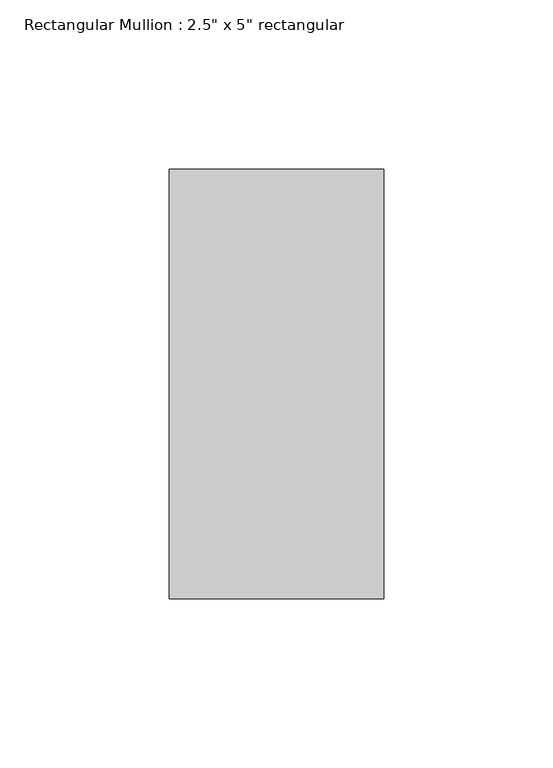
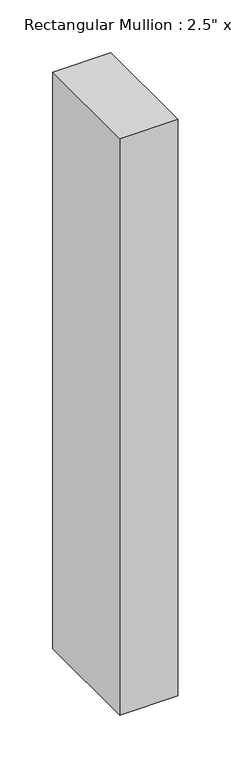
"""IFC4 building model written with IfcOpenShell, lengths in millimetres: member geometry."""

from ifc_helpers import new_model, si_unit, frame, origin, place, context, project, spatial, polyline, outline, extrude, source, transform, mapped, element, save


def member_2ee2964b(model_context):
    return source(origin(), model_context, "Body", "SweptSolid", [
        extrude(outline(polyline([(31.75, 63.5), (31.75, -63.5), (-31.75, -63.5), (-31.75, 63.5), (31.75, 63.5)])), frame((0.0, 0.0, -666.75), z_axis=(0.0, 0.0, 1.0), x_axis=(1.0, 0.0, 0.0)), (0.0, 0.0, 1.0), 666.75),
    ])


if __name__ == "__main__":
    model = new_model("IFC4")
    model_context = context("Model", 3, world=origin())
    ifc_project = project(units=[si_unit("LENGTHUNIT", "METRE", prefix="MILLI")], contexts=[model_context])
    site = spatial("IfcSite", under=ifc_project)
    building = spatial("IfcBuilding", under=site)
    placement = place(None, origin())
    member_shape = member_2ee2964b(model_context)
    element("IfcMember", 1, ObjectType="Rectangular Mullion : 2.5\" x 5\" rectangular", at=placement, inside=building, context=model_context, shape_type="MappedRepresentation", body=[
        mapped(member_shape, transform((0.0, 0.0, 0.0), x_axis=(1.0, 0.0, 0.0), y_axis=(0.0, 1.0, 0.0), z_axis=(0.0, 0.0, 1.0))),
    ])
    save(model, "model.ifc")

# Revit data of these elements
# Type "Rectangular Mullion : 2.5\" x 5\" rectangular"
#   built-in parameter 1007304 = 0.416667 (stored number, unit not read)
#   built-in parameter 1007301 = 0.104167 (stored number, unit not read)
#   built-in parameter 1007300 = 0.104167 (stored number, unit not read)
# Element 1 (IfcMember, "Rectangular Mullion : 2.5\" x 5\" rectangular")
#   Materials on its faces: "Aluminum"
# Materials
#   "Aluminum": class "Metal", colour RGB 247 247 247, transparency 0, Description = "Aluminum 6061", Cost = 0
